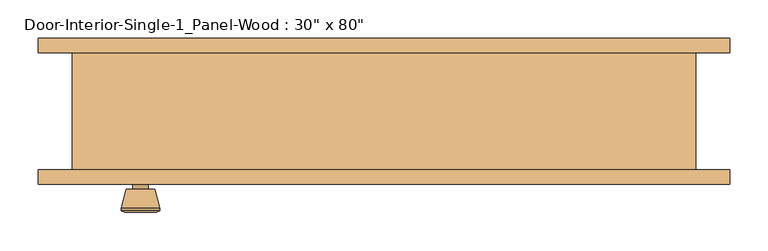
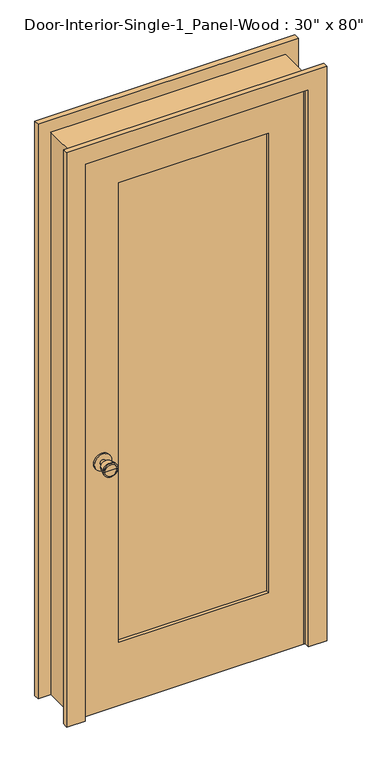
"""IFC4 building model written with IfcOpenShell, lengths in millimetres: door geometry."""

from ifc_helpers import new_model, si_unit, point, frame, frame_2d, origin, place, context, project, spatial, polyline, circle_curve, trimmed, segment, composite_curve, outline, extrude, faceted_brep, source, transform, mapped, element, save
from ifc_brep_helpers import plane_surface, cylinder_surface, revolved_surface, advanced_brep


def door_7bbed545(model_context):
    return source(origin(), model_context, "Body", "SolidModel", [
        advanced_brep(
        [(-317.5, -32.1, 914.4), (-327.5, -32.1, 914.4), (-307.5, -32.1, 914.4), (-297.0241324, 16.9, 914.4), (-337.9758676, 16.9, 914.4), (-317.5, 16.9, 914.4), (-292.5, 15.0721319, 914.4), (-342.5, 15.0721319, 914.4), (-292.5, 11.6084537, 914.4), (-342.5, 11.6084537, 914.4), (-298.863764, -13.1, 914.4), (-336.136236, -13.1, 914.4), (-307.5, -13.1, 914.4), (-327.5, -13.1, 914.4)],
        [
            (0, 1),
            (1, 2, circle_curve(frame((-317.5, -32.1, 914.4), z_axis=(0.0, -1.0, 0.0), x_axis=(-1.0, 0.0, 0.0)), 10.0)),
            (2, 0),
            (2, 1, circle_curve(frame((-317.5, -32.1, 914.4), z_axis=(0.0, -1.0, 0.0), x_axis=(-1.0, 0.0, 0.0)), 10.0)),
            (3, 4, circle_curve(frame((-317.5, 16.9, 914.4), z_axis=(0.0, 1.0, 0.0), x_axis=(-1.0, 0.0, 0.0)), 20.4758676)),
            (4, 5),
            (5, 3),
            (4, 3, circle_curve(frame((-317.5, 16.9, 914.4), z_axis=(0.0, 1.0, 0.0), x_axis=(-1.0, 0.0, 0.0)), 20.4758676)),
            (6, 7, circle_curve(frame((-317.5, 15.0721319, 914.4), z_axis=(0.0, 1.0, 0.0), x_axis=(-1.0, 0.0, 0.0)), 25.0)),
            (7, 4),
            (3, 6),
            (7, 6, circle_curve(frame((-317.5, 15.0721319, 914.4), z_axis=(0.0, 1.0, 0.0), x_axis=(-1.0, 0.0, 0.0)), 25.0)),
            (8, 9, circle_curve(frame((-317.5, 11.6084537, 914.4), z_axis=(0.0, 1.0, 0.0), x_axis=(-1.0, 0.0, 0.0)), 25.0)),
            (9, 7),
            (6, 8),
            (9, 8, circle_curve(frame((-317.5, 11.6084537, 914.4), z_axis=(0.0, 1.0, 0.0), x_axis=(-1.0, 0.0, 0.0)), 25.0)),
            (10, 11, circle_curve(frame((-317.5, -13.1, 914.4), z_axis=(0.0, 1.0, 0.0), x_axis=(-1.0, 0.0, 0.0)), 18.636236)),
            (11, 9),
            (8, 10),
            (11, 10, circle_curve(frame((-317.5, -13.1, 914.4), z_axis=(0.0, 1.0, 0.0), x_axis=(-1.0, 0.0, 0.0)), 18.636236)),
            (12, 13, circle_curve(frame((-317.5, -13.1, 914.4), z_axis=(0.0, 1.0, 0.0), x_axis=(-1.0, 0.0, 0.0)), 10.0)),
            (13, 11),
            (10, 12),
            (13, 12, circle_curve(frame((-317.5, -13.1, 914.4), z_axis=(0.0, 1.0, 0.0), x_axis=(-1.0, 0.0, 0.0)), 10.0)),
            (1, 13),
            (12, 2),
        ],
        [
            plane_surface(frame((-317.5, -32.1, 914.4), z_axis=(0.0, -1.0, 0.0), x_axis=(-1.0, 0.0, 0.0))),
            plane_surface(frame((-317.5, 16.9, 914.4), z_axis=(0.0, 1.0, 0.0), x_axis=(-1.0, 0.0, 0.0))),
            revolved_surface(polyline([(-337.9758676, 16.9, 914.4), (-342.5, 15.0721319, 914.4)]), (-317.5, -32.1, 914.4), (0.0, -1.0, 0.0)),
            cylinder_surface(frame((-317.5, -32.1, 914.4), z_axis=(0.0, -1.0, 0.0), x_axis=(-1.0, 0.0, 0.0)), 25.0),
            revolved_surface(polyline([(-342.5, 11.6084537, 914.4), (-336.136236, -13.1, 914.4)]), (-317.5, -32.1, 914.4), (0.0, -1.0, 0.0)),
            plane_surface(frame((-317.5, -13.1, 914.4), z_axis=(0.0, -1.0, 0.0), x_axis=(-1.0, 0.0, 0.0))),
            cylinder_surface(frame((-317.5, -32.1, 914.4), z_axis=(0.0, -1.0, 0.0), x_axis=(-1.0, 0.0, 0.0)), 10.0),
        ],
        [
            (0, [[1, 2, 3]]),
            (0, [[-3, 4, -1]]),
            (1, [[5, 6, 7]]),
            (1, [[8, -7, -6]]),
            (2, [[9, 10, -5, 11]]),
            (2, [[12, -11, -8, -10]]),
            (3, [[13, 14, -9, 15]]),
            (3, [[16, -15, -12, -14]]),
            (4, [[17, 18, -13, 19]]),
            (4, [[20, -19, -16, -18]]),
            (5, [[21, 22, -17, 23]]),
            (5, [[24, -23, -20, -22]]),
            (6, [[-2, 25, -21, 26]]),
            (6, [[-4, -26, -24, -25]]),
        ],
    ),
        extrude(outline(composite_curve([segment(trimmed(circle_curve(frame_2d((914.4, -317.5)), 30.0), [point((914.4, -347.5))], [point((914.4, -287.5))], False, "CARTESIAN"), True, "CONTINUOUS"), segment(trimmed(circle_curve(frame_2d((914.4, -317.5)), 30.0), [point((914.4, -287.5))], [point((914.4, -347.5))], False, "CARTESIAN"), True, "CONTINUOUS")], self_intersect=False)), frame((0.0, -38.1, 0.0), z_axis=(0.0, 1.0, 0.0), x_axis=(0.0, 0.0, 1.0)), (0.0, 0.0, 1.0), 6.0),
        advanced_brep(
        [(-317.5, -79.025, 914.4), (-307.5, -79.025, 914.4), (-327.5, -79.025, 914.4), (-297.0241324, -128.025, 914.4), (-317.5, -128.025, 914.4), (-337.9758676, -128.025, 914.4), (-292.5, -126.1971319, 914.4), (-342.5, -126.1971319, 914.4), (-292.5, -122.7334537, 914.4), (-342.5, -122.7334537, 914.4), (-298.863764, -98.025, 914.4), (-336.136236, -98.025, 914.4), (-307.5, -98.025, 914.4), (-327.5, -98.025, 914.4)],
        [
            (0, 1),
            (1, 2, circle_curve(frame((-317.5, -79.025, 914.4), z_axis=(0.0, 1.0, 0.0), x_axis=(-1.0, 0.0, 0.0)), 10.0)),
            (2, 0),
            (2, 1, circle_curve(frame((-317.5, -79.025, 914.4), z_axis=(0.0, 1.0, 0.0), x_axis=(-1.0, 0.0, 0.0)), 10.0)),
            (3, 4),
            (4, 5),
            (5, 3, circle_curve(frame((-317.5, -128.025, 914.4), z_axis=(0.0, -1.0, 0.0), x_axis=(-1.0, 0.0, 0.0)), 20.4758676)),
            (3, 5, circle_curve(frame((-317.5, -128.025, 914.4), z_axis=(0.0, -1.0, 0.0), x_axis=(-1.0, 0.0, 0.0)), 20.4758676)),
            (6, 3),
            (5, 7),
            (7, 6, circle_curve(frame((-317.5, -126.1971319, 914.4), z_axis=(0.0, -1.0, 0.0), x_axis=(-1.0, 0.0, 0.0)), 25.0)),
            (6, 7, circle_curve(frame((-317.5, -126.1971319, 914.4), z_axis=(0.0, -1.0, 0.0), x_axis=(-1.0, 0.0, 0.0)), 25.0)),
            (8, 6),
            (7, 9),
            (9, 8, circle_curve(frame((-317.5, -122.7334537, 914.4), z_axis=(0.0, -1.0, 0.0), x_axis=(-1.0, 0.0, 0.0)), 25.0)),
            (8, 9, circle_curve(frame((-317.5, -122.7334537, 914.4), z_axis=(0.0, -1.0, 0.0), x_axis=(-1.0, 0.0, 0.0)), 25.0)),
            (10, 8),
            (9, 11),
            (11, 10, circle_curve(frame((-317.5, -98.025, 914.4), z_axis=(0.0, -1.0, 0.0), x_axis=(-1.0, 0.0, 0.0)), 18.636236)),
            (10, 11, circle_curve(frame((-317.5, -98.025, 914.4), z_axis=(0.0, -1.0, 0.0), x_axis=(-1.0, 0.0, 0.0)), 18.636236)),
            (12, 10),
            (11, 13),
            (13, 12, circle_curve(frame((-317.5, -98.025, 914.4), z_axis=(0.0, -1.0, 0.0), x_axis=(-1.0, 0.0, 0.0)), 10.0)),
            (12, 13, circle_curve(frame((-317.5, -98.025, 914.4), z_axis=(0.0, -1.0, 0.0), x_axis=(-1.0, 0.0, 0.0)), 10.0)),
            (1, 12),
            (13, 2),
        ],
        [
            plane_surface(frame((-317.5, -79.025, 914.4), z_axis=(0.0, 1.0, 0.0), x_axis=(-1.0, 0.0, 0.0))),
            plane_surface(frame((-317.5, -128.025, 914.4), z_axis=(0.0, -1.0, 0.0), x_axis=(-1.0, 0.0, 0.0))),
            revolved_surface(polyline([(-337.9758676, -128.025, 914.4), (-342.5, -126.1971319, 914.4)]), (-317.5, -79.025, 914.4), (0.0, 1.0, 0.0)),
            cylinder_surface(frame((-317.5, -79.025, 914.4), z_axis=(0.0, 1.0, 0.0), x_axis=(-1.0, 0.0, 0.0)), 25.0),
            revolved_surface(polyline([(-342.5, -122.7334537, 914.4), (-336.136236, -98.025, 914.4)]), (-317.5, -79.025, 914.4), (0.0, 1.0, 0.0)),
            plane_surface(frame((-317.5, -98.025, 914.4), z_axis=(0.0, 1.0, 0.0), x_axis=(-1.0, 0.0, 0.0))),
            cylinder_surface(frame((-317.5, -79.025, 914.4), z_axis=(0.0, 1.0, 0.0), x_axis=(-1.0, 0.0, 0.0)), 10.0),
        ],
        [
            (0, [[1, 2, 3]]),
            (0, [[-3, 4, -1]]),
            (1, [[5, 6, 7]]),
            (1, [[-6, -5, 8]]),
            (2, [[9, -7, 10, 11]]),
            (2, [[-10, -8, -9, 12]]),
            (3, [[13, -11, 14, 15]]),
            (3, [[-14, -12, -13, 16]]),
            (4, [[17, -15, 18, 19]]),
            (4, [[-18, -16, -17, 20]]),
            (5, [[21, -19, 22, 23]]),
            (5, [[-22, -20, -21, 24]]),
            (6, [[25, -23, 26, -2]]),
            (6, [[-26, -24, -25, -4]]),
        ],
    ),
        extrude(outline(composite_curve([segment(trimmed(circle_curve(frame_2d((914.4, -317.5)), 30.0), [point((914.4, -347.5))], [point((914.4, -287.5))], False, "CARTESIAN"), True, "CONTINUOUS"), segment(trimmed(circle_curve(frame_2d((914.4, -317.5)), 30.0), [point((914.4, -287.5))], [point((914.4, -347.5))], False, "CARTESIAN"), True, "CONTINUOUS")], self_intersect=False)), frame((0.0, -79.025, 0.0), z_axis=(0.0, 1.0, 0.0), x_axis=(0.0, 0.0, 1.0)), (0.0, 0.0, 1.0), 6.0),
        extrude(outline(polyline([(260.35, -49.7416667), (260.35, -61.3833333), (-260.35, -61.3833333), (-260.35, -49.7416667), (260.35, -49.7416667)])), frame((0.0, 0.0, 231.775), z_axis=(0.0, 0.0, 1.0), x_axis=(1.0, 0.0, 0.0)), (0.0, 0.0, 1.0), 1681.1625),
        extrude(outline(polyline([(2032.0, -381.0), (0.0, -381.0), (0.0, 381.0), (2032.0, 381.0), (2032.0, -381.0)]), holes=[polyline([(1912.9375, -260.35), (1912.9375, 260.35), (231.775, 260.35), (231.775, -260.35), (1912.9375, -260.35)])]), frame((0.0, -73.025, 0.0), z_axis=(0.0, 1.0, 0.0), x_axis=(0.0, 0.0, 1.0)), (0.0, 0.0, 1.0), 34.925),
        faceted_brep([(406.4, -73.025, 0.0), (381.0, -73.025, 0.0), (381.0, -38.1, 0.0), (368.3, -38.1, 0.0), (368.3, -3.175, 0.0), (381.0, -3.175, 0.0), (381.0, 79.375, 0.0), (406.4, 79.375, 0.0), (406.4, 79.375, 2057.4), (406.4, -73.025, 2057.4), (381.0, 79.375, 2032.0), (-381.0, 79.375, 2032.0), (-381.0, 79.375, 0.0), (-406.4, 79.375, 0.0), (-406.4, 79.375, 2057.4), (381.0, -3.175, 2032.0), (368.3, -3.175, 2019.3), (-368.3, -3.175, 2019.3), (-368.3, -3.175, 0.0), (-381.0, -3.175, 0.0), (-381.0, -3.175, 2032.0), (368.3, -38.1, 2019.3), (381.0, -38.1, 2032.0), (-381.0, -38.1, 2032.0), (-381.0, -38.1, 0.0), (-368.3, -38.1, 0.0), (-368.3, -38.1, 2019.3), (381.0, -73.025, 2032.0), (-406.4, -73.025, 2057.4), (-406.4, -73.025, 0.0), (-381.0, -73.025, 0.0), (-381.0, -73.025, 2032.0)], [[[0, 1, 2, 3, 4, 5, 6, 7]], [[7, 8, 9, 0]], [[6, 10, 11, 12, 13, 14, 8, 7]], [[5, 15, 10, 6]], [[4, 16, 17, 18, 19, 20, 15, 5]], [[3, 21, 16, 4]], [[2, 22, 23, 24, 25, 26, 21, 3]], [[1, 27, 22, 2]], [[0, 9, 28, 29, 30, 31, 27, 1]], [[8, 14, 28, 9]], [[15, 20, 11, 10]], [[21, 26, 17, 16]], [[27, 31, 23, 22]], [[29, 13, 12, 19, 18, 25, 24, 30]], [[14, 13, 29, 28]], [[20, 19, 12, 11]], [[26, 25, 18, 17]], [[31, 30, 24, 23]]]),
        extrude(outline(polyline([(0.0, 450.85), (2101.85, 450.85), (2101.85, -450.85), (0.0, -450.85), (0.0, -387.35), (2038.35, -387.35), (2038.35, 387.35), (0.0, 387.35), (0.0, 450.85)])), frame((0.0, 79.375, 0.0), z_axis=(0.0, 1.0, 0.0), x_axis=(0.0, 0.0, 1.0)), (0.0, 0.0, 1.0), 19.05),
        extrude(outline(polyline([(0.0, 450.85), (2101.85, 450.85), (2101.85, -450.85), (0.0, -450.85), (0.0, -387.35), (2038.35, -387.35), (2038.35, 387.35), (0.0, 387.35), (0.0, 450.85)])), frame((0.0, -92.075, 0.0), z_axis=(0.0, 1.0, 0.0), x_axis=(0.0, 0.0, 1.0)), (0.0, 0.0, 1.0), 19.05),
    ])


if __name__ == "__main__":
    model = new_model("IFC4")
    model_context = context("Model", 3, world=origin())
    ifc_project = project(units=[si_unit("LENGTHUNIT", "METRE", prefix="MILLI")], contexts=[model_context])
    site = spatial("IfcSite", under=ifc_project)
    building = spatial("IfcBuilding", under=site)
    placement = place(None, origin())
    door_shape = door_7bbed545(model_context)
    element("IfcDoor", 1, ObjectType="Door-Interior-Single-1_Panel-Wood : 30\" x 80\"", at=placement, inside=building, context=model_context, shape_type="MappedRepresentation", body=[
        mapped(door_shape, transform((0.0, 0.0, 0.0), x_axis=(1.0, 0.0, 0.0), y_axis=(0.0, 1.0, 0.0), z_axis=(0.0, 0.0, 1.0))),
    ])
    save(model, "model.ifc")

# Revit data of these elements
# Type "Door-Interior-Single-1_Panel-Wood : 30\" x 80\""
#   Type Mark = "10"
#   Assembly Code = "C1020300"
#   Analytic Construction = "Wooden"
#   Top Rail = 0' - 4 11/16"
#   Thickness = 0' - 1 3/8"
#   Thermal Resistance (R) = 2.5876 (h·ft²·°F)/BTU
#   Swing Angle [instance default] = 90.00°
#   Stiles = 0' - 4 3/4"
#   Rough Width = 2' - 8"
#   Rough Height = 6' - 9"
#   Height = 6' - 8"
#   Width = 2' - 6"
#   Heat Transfer Coefficient (U) = 0.3865 BTU/(h·ft²·°F)
#   Bottom Rail = 0' - 9 1/8"
#   Trim Material = Cherry
#   Panel Material = Cherry
#   Frame Material = Cherry
#   Door Handle Material = Aluminum
#   Visual Light Transmittance = 0
#   Solar Heat Gain Coefficient = 0
#   Wall Closure = (empty or 0)
#   Function = (empty or 0)
# Element 1 (IfcDoor, "Door-Interior-Single-1_Panel-Wood : 30\" x 80\"")
#   Materials on its faces: "Cherry", "Aluminum"
# Materials
#   "Cherry": class "Wood", colour RGB 226 177 128, transparency 0, Description = "Prunus Serotina", Cost = 0
#   "Aluminum": class "Metal", colour RGB 247 247 247, transparency 0, Description = "Aluminum 6061", Cost = 0
